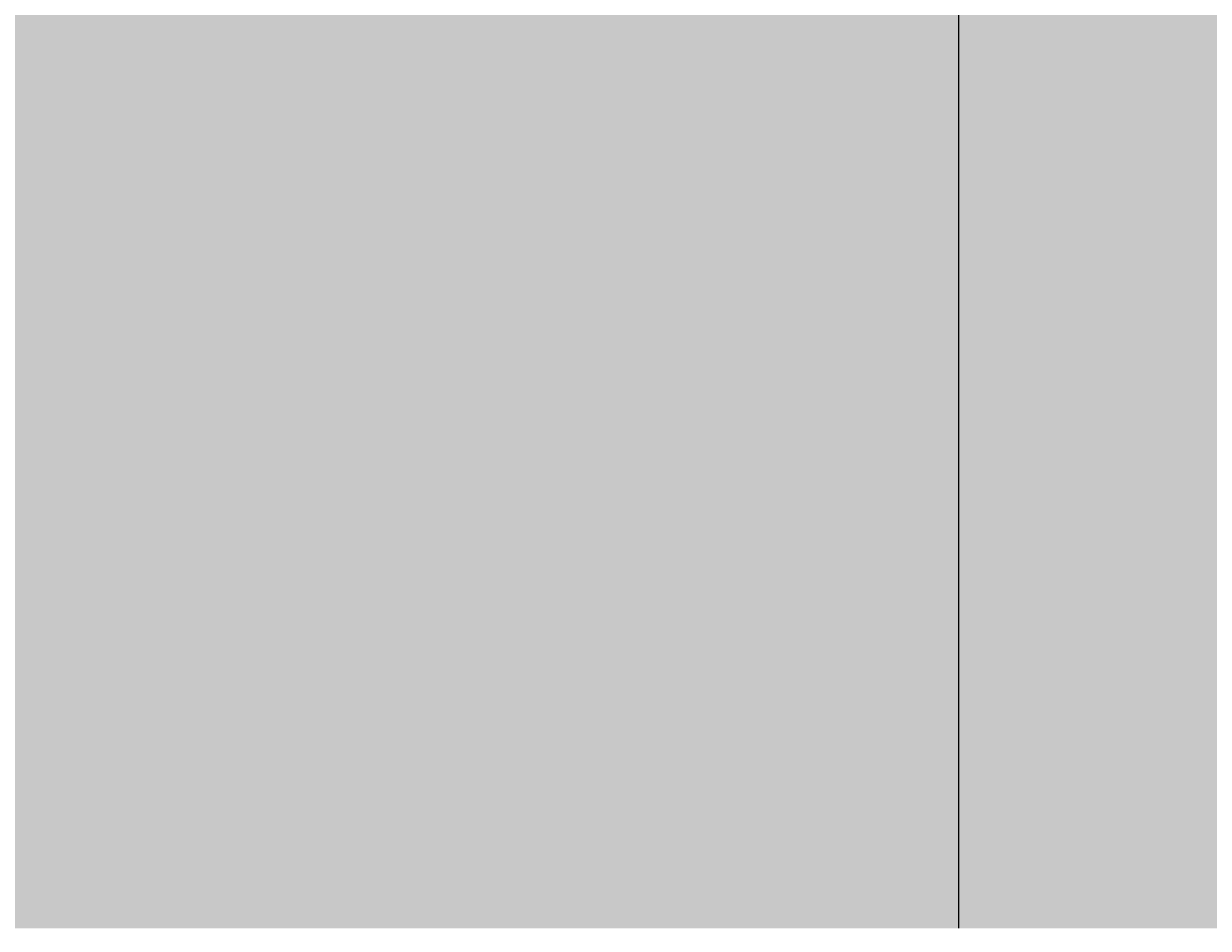
# Model space of a CAD drawing. Units: inches. Extents: x 84 to 1044, y -280 to 906.
# Tile 59 of 105: x 412 to 440, y 709 to 731. Entities that reach past the tile are written whole.
import ezdxf

# ---------------------------------------------------------------- set-up
doc = ezdxf.new("R2010")
doc.units = ezdxf.units.IN
doc.layers.add('A-ANNO-DIMS', color=2, linetype='Continuous', lineweight=18)
doc.layers.add('L-HRDS', color=32, linetype='Continuous', lineweight=18)
doc.layers.add('L-PLNT-PATT', color=9, linetype='Continuous', lineweight=9, true_color=0xafd9aa)
doc.styles.get("Standard").update_dxf_attribs({"font": 'arial.ttf'})
doc.dimstyles.get("Standard").update_dxf_attribs({"dimtxt": 0.18, "dimasz": 0.18, "dimexe": 0.18, "dimexo": 0.0625, "dimgap": 0.09, "dimtad": 0, "dimtih": 1, "dimtoh": 1, "dimdec": 4, "dimzin": 0, "dimdsep": 46, "dimtxsty": 'Standard', "dimcen": 0.09, "dimadec": 0, "dimazin": 0, "dimtfac": 1, "dimtdec": 4, "dimtofl": 0, "dimtmove": 0, "dimatfit": 3, "dimfxl": 1, "dimtolj": 1, "dimtzin": 0, "dimarcsym": 0})

# ---------------------------------------------------------------- blocks, each defined once
blk = doc.blocks.new('*D62')
at = {"layer": 'A-ANNO-DIMS', "color": 0, "lineweight": -2, "transparency": 16777216}
for p, q in [((203.179, 709.183), (203.179, 905.9)), ((896.074, 400.183), (896.074, 905.9)), ((203.359, 905.72), (549.232, 905.72)), ((895.894, 905.72), (550.021, 905.72))]:
    blk.add_line(p, q, dxfattribs=at)
at = {"layer": 'A-ANNO-DIMS', "color": 0, "transparency": 16777216}
for points in [[(203.359, 905.75), (203.359, 905.69), (203.179, 905.72)], [(895.894, 905.75), (895.894, 905.69), (896.074, 905.72)]]:
    blk.add_solid(points, dxfattribs=at)
at = {"layer": 'Defpoints', "color": 0, "transparency": 16777216}
for p in [(896.074, 905.72), (203.179, 709.12), (896.074, 400.12)]:
    blk.add_point(p, dxfattribs=at)
at = {"layer": 'A-ANNO-DIMS', "color": 0, "transparency": 16777216, "insert": (549.627, 905.72), "char_height": 0.18, "attachment_point": 5}
blk.add_mtext('\\A1;692.9', dxfattribs=at)

msp = doc.modelspace()

# ---------------------------------------------------------------- hatches: boundary and pattern name
at = {"layer": 'L-PLNT-PATT', "transparency": 33554597}
h = msp.add_hatch(color=256, dxfattribs=at)
h.dxf.hatch_style = 1
h.paths.add_polyline_path([(434.074, 769.12), (386.074, 769.12), (386.074, 709.12), (434.074, 709.12)])
h.paths.add_polyline_path([(896.074, 847.12), (434.074, 847.12), (434.074, 769.12), (434.074, 709.12), (470.074, 709.12), (506.074, 709.12), (572.074, 709.12), (608.074, 709.12), (698.074, 709.12), (770.074, 709.12), (833.074, 709.12), (896.074, 709.12)])
h.paths.add_polyline_path([(983.074, 847.12), (896.074, 847.12), (896.074, 709.12), (896.074, 547.12), (932.074, 547.12), (983.074, 547.12)])
h.paths.add_polyline_path([(983.074, 547.12), (932.074, 547.12), (932.074, 265.12), (983.074, 265.12)])
h.paths.add_polyline_path([(203.179, 646.12), (203.179, 709.12), (203.179, 745.12), (143.179, 745.12), (143.179, 271.12), (203.179, 271.12), (203.179, 274.12), (203.179, 310.12), (203.179, 574.12)])

# ---------------------------------------------------------------- linework, layer by layer
at = {"layer": 'L-HRDS'}
msp.add_line((434.074, 769.12), (434.074, 709.12), dxfattribs=at)

# ---------------------------------------------------------------- dimensions: what is measured, and where the dimension line sits
at = {"layer": 'A-ANNO-DIMS'}
dim = msp.add_linear_dim(base=(896.074, 905.72), p1=(203.179, 709.12), p2=(896.074, 400.12), dimstyle='Standard', override={"dimdec": 1, "dimlfac": 1, "dimrnd": 0, "dimzin": 0, "dimdsep": 46, "dimlunit": 2}, dxfattribs=at)
dim.commit()
dim.dimension.update_dxf_attribs({"geometry": '*D62', "text_midpoint": (549.627, 905.72)})

doc.saveas('drawing.dxf')
